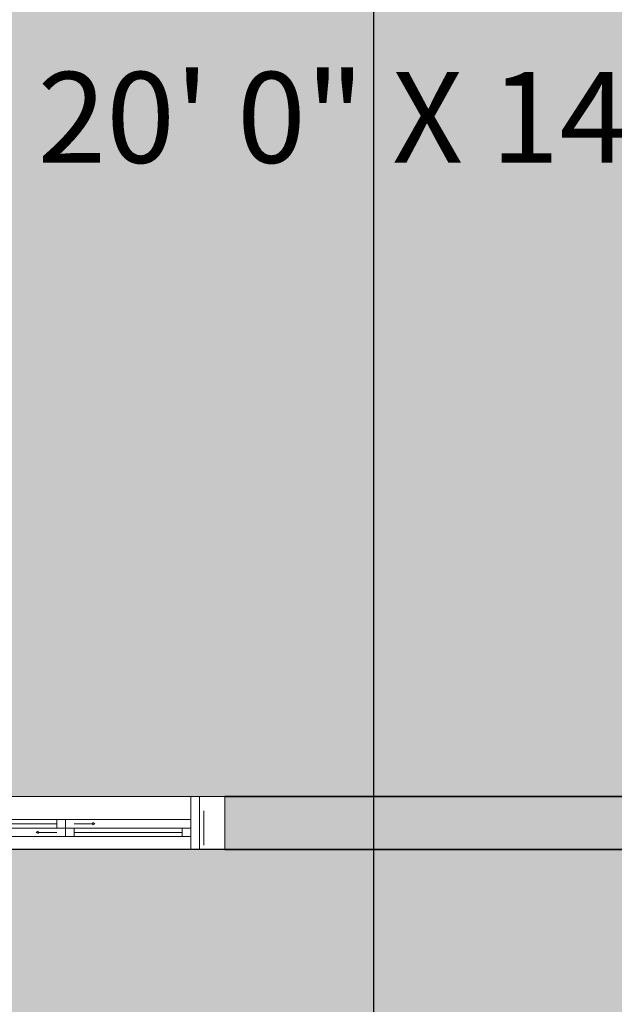
# Model space of a CAD drawing. Units: inches. Extents: x 1704 to 6393, y -157 to 1172.
# Tile 32 of 122: x 2398 to 2488, y 67 to 215. Entities that reach past the tile are written whole.
import ezdxf

# ---------------------------------------------------------------- set-up
doc = ezdxf.new("R2010")
doc.units = ezdxf.units.IN
doc.header["$MEASUREMENT"] = 0
for name, color, linetype, lineweight in [('A-ANNO-DIMS', 7, 'Continuous', 13), ('A-WALL-PATT', 7, 'Continuous', 13), ('WALLS', 7, 'Continuous', 35), ('WINDOWS', 2, 'Continuous', 18)]:
    doc.layers.add(name, color=color, linetype=linetype, lineweight=lineweight)
doc.layers.add('A-FLOR-PATT', color=7, linetype='Continuous', lineweight=13, true_color=0xf2f2f2)
doc.layers.add('L-HRDS-PATT', color=9, linetype='Continuous', lineweight=13, true_color=0xc5c1ba)
doc.styles.get("Standard").update_dxf_attribs({"font": 'arial.ttf'})
doc.dimstyles.get("Standard").update_dxf_attribs({"dimtxt": 6, "dimasz": 2, "dimexe": 0.18, "dimexo": 0.0625, "dimgap": 0.09, "dimtad": 0, "dimtih": 1, "dimtoh": 1, "dimdec": 1, "dimzin": 0, "dimdsep": 46, "dimlunit": 3, "dimtxsty": 'Standard', "dimblk": 'ARCHTICK', "dimcen": 0.09, "dimadec": 0, "dimazin": 0, "dimtfac": 1, "dimtdec": 1, "dimtofl": 0, "dimtmove": 0, "dimatfit": 3, "dimfxl": 1, "dimtolj": 1, "dimtzin": 0, "dimarcsym": 0})

# ---------------------------------------------------------------- blocks, each defined once
blk = doc.blocks.new('WIN-SLIDER-48')
for p, q in [((3.83, 8), (0, 8)), ((5.13, 8), (42.87, 8)), ((44.17, 8), (48, 8)), ((3.18, 5.86), (3.18, 0.65)), ((6.43, 4.55), (22.7, 4.55)), ((24, 4.55), (42.87, 4.55)), ((44.82, 5.86), (44.82, 0.65)), ((6.43, 3.9), (22.7, 3.9)), ((6.43, 3.25), (22.7, 3.25)), ((25.3, 3.9), (28.1, 3.9)), ((25.3, 3.25), (41.56, 3.25)), ((24, 1.95), (5.13, 1.95)), ((22.7, 2.6), (19.9, 2.6)), ((25.3, 2.6), (41.56, 2.6)), ((25.3, 1.95), (41.56, 1.95)), ((3.83, 0), (0, 0)), ((5.13, 0), (42.87, 0)), ((44.17, 0), (48, 0))]:
    blk.add_line(p, q)
for points in [[(5.13, 0), (3.83, 0), (3.83, 8), (5.13, 8)], [(42.87, 0), (44.17, 0), (44.17, 8), (42.87, 8)], [(5.13, 3.25), (6.43, 3.25), (6.43, 4.55), (5.13, 4.55)], [(22.7, 3.25), (24, 3.25), (24, 4.55), (22.7, 4.55)], [(24, 1.95), (25.3, 1.95), (25.3, 3.25), (24, 3.25)], [(28.43, 3.9), (28.1, 4.1), (28.1, 3.71)], [(41.56, 1.95), (42.87, 1.95), (42.87, 3.25), (41.56, 3.25)], [(19.57, 2.6), (19.9, 2.8), (19.9, 2.41)]]:
    blk.add_lwpolyline(points, close=True)
blk = doc.blocks.new('_ArchTick')
at = {"color": 0, "linetype": 'ByBlock', "const_width": 0.15}
blk.add_lwpolyline([(-0.5, -0.5), (0.5, 0.5)], dxfattribs=at)
blk = doc.blocks.new('*D93')
at = {"layer": 'A-ANNO-DIMS', "color": 0, "lineweight": -2, "transparency": 16777216}
for p, q in [((2605.29, 895.21), (1829.7, 895.21)), ((1829.88, 895.21), (1829.88, 495.87)), ((1829.88, 90.21), (1829.88, 489.56)), ((2605.29, 90.21), (1829.7, 90.21))]:
    blk.add_line(p, q, dxfattribs=at)
at = {"layer": 'Defpoints', "color": 0, "lineweight": -3, "transparency": 16777216}
for p in [(2605.35, 895.21), (1829.88, 90.21), (2605.35, 90.21)]:
    blk.add_point(p, dxfattribs=at)
at = {"layer": 'A-ANNO-DIMS', "color": 0, "lineweight": -2, "transparency": 16777216, "xscale": 2, "yscale": 2, "zscale": 2}
for p, rotation in [((1829.88, 895.21), 90), ((1829.88, 90.21), 270)]:
    blk.add_blockref('_ArchTick', p, dxfattribs=dict(at, rotation=rotation))
at = {"layer": 'A-ANNO-DIMS', "color": 0, "transparency": 16777216, "insert": (1829.88, 492.71), "char_height": 6, "attachment_point": 5}
blk.add_mtext('\\A1;805', dxfattribs=at)
blk = doc.blocks.new('*D105')
at = {"layer": 'A-ANNO-DIMS', "color": 0, "lineweight": -2, "transparency": 16777216}
for p, q in [((2451.74, 615.15), (2451.74, -64.97)), ((2547.35, 615.15), (2547.35, -64.97)), ((2451.74, -64.79), (2489.91, -64.79)), ((2547.35, -64.79), (2509.18, -64.79))]:
    blk.add_line(p, q, dxfattribs=at)
at = {"layer": 'Defpoints', "color": 0, "lineweight": -3, "transparency": 16777216}
for p in [(2451.74, 615.21), (2547.35, 615.21), (2547.35, -64.79)]:
    blk.add_point(p, dxfattribs=at)
at = {"layer": 'A-ANNO-DIMS', "color": 0, "lineweight": -2, "transparency": 16777216, "xscale": 2, "yscale": 2, "zscale": 2, "rotation": 180}
blk.add_blockref('_ArchTick', (2451.74, -64.79), dxfattribs=at)
at = {"layer": 'A-ANNO-DIMS', "color": 0, "lineweight": -2, "transparency": 16777216, "xscale": 2, "yscale": 2, "zscale": 2}
blk.add_blockref('_ArchTick', (2547.35, -64.79), dxfattribs=at)
at = {"layer": 'A-ANNO-DIMS', "color": 0, "transparency": 16777216, "insert": (2499.54, -64.79), "char_height": 6, "attachment_point": 5}
blk.add_mtext('\\A1;95.61', dxfattribs=at)

msp = doc.modelspace()

# ---------------------------------------------------------------- hatches: boundary and pattern name
at = {"layer": 'A-FLOR-PATT', "transparency": 33554528}
h = msp.add_hatch(color=256, dxfattribs=at)
h.dxf.hatch_style = 1
h.paths.add_polyline_path([(2325.349, 863.213), (2325.349, 887.213), (2263.349, 887.213), (2167.349, 887.213), (2081.349, 887.213), (2081.349, 719.213), (2277.349, 719.213), (2277.349, 711.213), (2277.349, 372.213), (2349.349, 372.213), (2381.349, 372.213), (2381.349, 364.213), (2353.349, 364.213), (2353.349, 270.213), (2381.349, 270.213), (2381.349, 266.213), (2357.349, 266.213), (2357.349, 98.213), (2381.349, 98.213), (2385.181, 98.213), (2386.482, 98.213), (2424.215, 98.213), (2425.516, 98.213), (2429.349, 98.213), (2597.349, 98.213), (2597.349, 146.213), (2597.349, 218.213), (2597.349, 266.213), (2423.349, 266.213), (2423.349, 270.213), (2473.349, 270.213), (2473.349, 294.213), (2477.349, 294.213), (2477.349, 270.213), (2547.349, 270.213), (2547.349, 364.213), (2477.349, 364.213), (2477.349, 318.213), (2473.349, 318.213), (2473.349, 364.213), (2423.349, 364.213), (2423.349, 372.213), (2469.349, 372.213), (2469.349, 459.213), (2469.349, 538.213), (2350.349, 538.213), (2350.349, 565.713), (2358.349, 565.713), (2358.349, 545.213), (2420.349, 545.213), (2420.349, 610.213), (2358.349, 610.213), (2358.349, 589.713), (2350.349, 589.713), (2350.349, 615.213), (2425.349, 615.213), (2425.349, 607.213), (2425.349, 546.213), (2469.349, 546.213), (2514.349, 546.213), (2514.349, 607.213), (2449.349, 607.213), (2449.349, 615.213), (2451.738, 615.213), (2451.738, 659.213), (2427.738, 659.213), (2427.738, 665.213), (2367.738, 665.213), (2367.738, 667.213), (2367.738, 711.213), (2325.349, 711.213), (2325.349, 719.213), (2325.349, 755.213), (2325.349, 763.213)])
h.paths.add_polyline_path([(2233.858, 822.533, -0.187247), (2233.858, 809.14), (2231.697, 808.804, 0.0848928), (2233.131, 814.486), (2230.424, 814.486, -0.1042581), (2228.553, 808.313), (2217.751, 807.156, -0.2222222), (2217.751, 824.517), (2228.553, 823.359, -0.1042581), (2230.424, 817.186), (2233.131, 817.186, 0.0848928), (2231.697, 822.868)], flags=16)
h.paths.add_polyline_path([(2213.621, 833.197), (2213.621, 798.475), (2156.048, 798.475), (2156.048, 833.197)], flags=16)
h.paths.add_polyline_path([(2203.932, 848.099), (2205.089, 837.296, -0.2222222), (2187.728, 837.296), (2188.885, 848.099, -0.1042581), (2195.058, 849.969), (2195.058, 852.676, 0.0848928), (2189.377, 851.242), (2189.712, 853.404, -0.187247), (2203.105, 853.404), (2203.44, 851.242, 0.0848928), (2197.759, 852.676), (2197.759, 849.969, -0.1042581)], flags=16)
h.paths.add_polyline_path([(2181.941, 837.296, -0.2222222), (2164.58, 837.296), (2165.737, 848.099, -0.1042581), (2171.91, 849.969), (2171.91, 852.676, 0.0848928), (2166.229, 851.242), (2166.564, 853.404, -0.187247), (2179.957, 853.404), (2180.292, 851.242, 0.0848928), (2174.611, 852.676), (2174.611, 849.969, -0.1042581), (2180.784, 848.099)], flags=16)
h.paths.add_polyline_path([(2205.089, 794.376), (2203.932, 783.574, -0.1042581), (2197.759, 781.703), (2197.759, 778.996, 0.0848928), (2203.44, 780.43), (2203.105, 778.269, -0.187247), (2189.712, 778.269), (2189.377, 780.43, 0.0848928), (2195.058, 778.996), (2195.058, 781.703, -0.1042581), (2188.885, 783.574), (2187.728, 794.376, -0.2222222)], flags=16)
h.paths.add_polyline_path([(2181.941, 794.376), (2180.784, 783.574, -0.1042581), (2174.611, 781.703), (2174.611, 778.996, 0.0848928), (2180.292, 780.43), (2179.957, 778.269, -0.187247), (2166.564, 778.269), (2166.229, 780.43, 0.0848928), (2171.91, 778.996), (2171.91, 781.703, -0.1042581), (2165.737, 783.574), (2164.58, 794.376, -0.2222222)], flags=16)
h.paths.add_polyline_path([(2151.918, 807.156), (2141.116, 808.313, -0.1042581), (2139.245, 814.486), (2136.539, 814.486, 0.0848928), (2137.972, 808.804), (2135.811, 809.14, -0.187247), (2135.811, 822.533), (2137.972, 822.868, 0.0848928), (2136.539, 817.186), (2139.245, 817.186, -0.1042581), (2141.116, 823.359), (2151.918, 824.517, -0.2222222)], flags=16)
h.paths.add_polyline_path([(2357.868, 363.41), (2358.814, 363.41, 0.7537605)], flags=16)
h.paths.add_polyline_path([(2372.241, 363.117), (2372.248, 363.117), (2372.248, 363.343), (2371.302, 363.343), (2371.302, 363.139, -1.3603913)], flags=16)
h.paths.add_polyline_path([(2371.309, 272.716), (2371.302, 272.716), (2371.302, 272.49), (2372.248, 272.49), (2372.248, 272.693, -1.3603913)], flags=16)
h.paths.add_polyline_path([(2357.875, 272.716), (2357.868, 272.716), (2357.868, 272.49), (2358.814, 272.49), (2358.814, 272.693, -1.3603913)], flags=16)
h.paths.add_polyline_path([(2353.769, 363.074), (2376.347, 363.074), (2376.347, 272.759), (2353.769, 272.759)], flags=16)
h.paths.add_polyline_path([(2354.772, 362.07), (2375.344, 362.07), (2375.344, 273.762), (2354.772, 273.762)], flags=0)
h.paths.add_polyline_path([(2357.868, 363.343), (2358.814, 363.343), (2358.814, 363.117), (2357.868, 363.117)], flags=16)
h.paths.add_polyline_path([(2359.288, 359.184), (2359.288, 360.063), (2370.828, 360.063), (2370.828, 359.184), (2374.332, 359.184), (2374.332, 358.464), (2372.835, 358.464), (2372.835, 357.541), (2374.332, 357.541), (2374.332, 356.82), (2372.835, 356.82), (2372.835, 355.898), (2374.332, 355.898), (2374.332, 355.177), (2372.835, 355.177), (2372.835, 354.254), (2374.332, 354.254), (2374.332, 353.534), (2372.835, 353.534), (2372.835, 352.611), (2374.332, 352.611), (2374.332, 351.89), (2372.835, 351.89), (2372.835, 350.968), (2374.332, 350.968), (2374.332, 350.247), (2372.835, 350.247), (2372.835, 349.324), (2374.332, 349.324), (2374.332, 348.604), (2372.835, 348.604), (2372.835, 347.681), (2374.332, 347.681), (2374.332, 346.96), (2372.835, 346.96), (2372.835, 346.038), (2374.332, 346.038), (2374.332, 345.317), (2372.835, 345.317), (2372.835, 344.395), (2374.332, 344.395), (2374.332, 343.674), (2372.835, 343.674), (2372.835, 342.751), (2374.332, 342.751), (2374.332, 342.03), (2372.835, 342.03), (2372.835, 341.108), (2374.332, 341.108), (2374.332, 340.387), (2372.835, 340.387), (2372.835, 339.465), (2374.332, 339.465), (2374.332, 338.744), (2372.835, 338.744), (2372.835, 337.821), (2374.332, 337.821), (2374.332, 337.1), (2372.835, 337.1), (2372.835, 336.178), (2374.332, 336.178), (2374.332, 335.457), (2372.835, 335.457), (2372.835, 334.535), (2374.332, 334.535), (2374.332, 333.814), (2372.835, 333.814), (2372.835, 332.891), (2374.332, 332.891), (2374.332, 332.171), (2372.835, 332.171), (2372.835, 331.248), (2374.332, 331.248), (2374.332, 330.527), (2372.835, 330.527), (2372.835, 329.605), (2374.332, 329.605), (2374.332, 328.884), (2372.835, 328.884), (2372.835, 327.961), (2374.332, 327.961), (2374.332, 327.241), (2372.835, 327.241), (2372.835, 326.318), (2374.332, 326.318), (2374.332, 325.597), (2372.835, 325.597), (2372.835, 324.675), (2374.332, 324.675), (2374.332, 323.954), (2372.835, 323.954), (2372.835, 323.031), (2374.332, 323.031), (2374.332, 322.311), (2372.835, 322.311), (2372.835, 321.388), (2374.332, 321.388), (2374.332, 320.667), (2372.835, 320.667), (2372.835, 319.745), (2374.332, 319.745), (2374.332, 319.024), (2372.835, 319.024), (2372.835, 318.102), (2374.332, 318.102), (2374.332, 317.381), (2372.835, 317.381), (2372.835, 316.458), (2374.332, 316.458), (2374.332, 315.737), (2372.835, 315.737), (2372.835, 314.815), (2374.332, 314.815), (2374.332, 314.094), (2372.835, 314.094), (2372.835, 313.172), (2374.332, 313.172), (2374.332, 312.451), (2372.835, 312.451), (2372.835, 311.528), (2374.332, 311.528), (2374.332, 310.807), (2372.835, 310.807), (2372.835, 309.885), (2374.332, 309.885), (2374.332, 309.164), (2372.835, 309.164), (2372.835, 308.242), (2374.332, 308.242), (2374.332, 307.521), (2372.835, 307.521), (2372.835, 306.598), (2374.332, 306.598), (2374.332, 305.878), (2372.835, 305.878), (2372.835, 304.955), (2374.332, 304.955), (2374.332, 304.234), (2372.835, 304.234), (2372.835, 303.312), (2374.332, 303.312), (2374.332, 302.591), (2372.835, 302.591), (2372.835, 301.668), (2374.332, 301.668), (2374.332, 300.948), (2372.835, 300.948), (2372.835, 300.025), (2374.332, 300.025), (2374.332, 299.304), (2372.835, 299.304), (2372.835, 298.382), (2374.332, 298.382), (2374.332, 297.661), (2372.835, 297.661), (2372.835, 296.738), (2374.332, 296.738), (2374.332, 296.018), (2372.835, 296.018), (2372.835, 295.095), (2374.332, 295.095), (2374.332, 294.374), (2372.835, 294.374), (2372.835, 293.452), (2374.332, 293.452), (2374.332, 292.731), (2372.835, 292.731), (2372.835, 291.809), (2374.332, 291.809), (2374.332, 291.088), (2372.835, 291.088), (2372.835, 290.165), (2374.332, 290.165), (2374.332, 289.444), (2372.835, 289.444), (2372.835, 288.522), (2374.332, 288.522), (2374.332, 287.801), (2372.835, 287.801), (2372.835, 286.879), (2374.332, 286.879), (2374.332, 286.158), (2372.835, 286.158), (2372.835, 285.235), (2374.332, 285.235), (2374.332, 284.514), (2372.835, 284.514), (2372.835, 283.592), (2374.332, 283.592), (2374.332, 282.871), (2372.835, 282.871), (2372.835, 281.949), (2374.332, 281.949), (2374.332, 281.228), (2372.835, 281.228), (2372.835, 280.305), (2374.332, 280.305), (2374.332, 279.585), (2372.835, 279.585), (2372.835, 278.662), (2374.332, 278.662), (2374.332, 277.941), (2372.835, 277.941), (2372.835, 277.019), (2374.332, 277.019), (2374.332, 276.298), (2370.828, 276.298), (2370.828, 275.769), (2359.288, 275.769), (2359.288, 276.298), (2355.784, 276.298), (2355.784, 277.019), (2357.281, 277.019), (2357.281, 277.941), (2355.784, 277.941), (2355.784, 278.662), (2357.281, 278.662), (2357.281, 279.585), (2355.784, 279.585), (2355.784, 280.305), (2357.281, 280.305), (2357.281, 281.228), (2355.784, 281.228), (2355.784, 281.949), (2357.281, 281.949), (2357.281, 282.871), (2355.784, 282.871), (2355.784, 283.592), (2357.281, 283.592), (2357.281, 284.514), (2355.784, 284.514), (2355.784, 285.235), (2357.281, 285.235), (2357.281, 286.158), (2355.784, 286.158), (2355.784, 286.879), (2357.281, 286.879), (2357.281, 287.801), (2355.784, 287.801), (2355.784, 288.522), (2357.281, 288.522), (2357.281, 289.444), (2355.784, 289.444), (2355.784, 290.165), (2357.281, 290.165), (2357.281, 291.088), (2355.784, 291.088), (2355.784, 291.809), (2357.281, 291.809), (2357.281, 292.731), (2355.784, 292.731), (2355.784, 293.452), (2357.281, 293.452), (2357.281, 294.374), (2355.784, 294.374), (2355.784, 295.095), (2357.281, 295.095), (2357.281, 296.018), (2355.784, 296.018), (2355.784, 296.738), (2357.281, 296.738), (2357.281, 297.661), (2355.784, 297.661), (2355.784, 298.382), (2357.281, 298.382), (2357.281, 299.304), (2355.784, 299.304), (2355.784, 300.025), (2357.281, 300.025), (2357.281, 300.948), (2355.784, 300.948), (2355.784, 301.668), (2357.281, 301.668), (2357.281, 302.591), (2355.784, 302.591), (2355.784, 303.312), (2357.281, 303.312), (2357.281, 304.234), (2355.784, 304.234), (2355.784, 304.955), (2357.281, 304.955), (2357.281, 305.878), (2355.784, 305.878), (2355.784, 306.598), (2357.281, 306.598), (2357.281, 307.521), (2355.784, 307.521), (2355.784, 308.242), (2357.281, 308.242), (2357.281, 309.164), (2355.784, 309.164), (2355.784, 309.885), (2357.281, 309.885), (2357.281, 310.807), (2355.784, 310.807), (2355.784, 311.528), (2357.281, 311.528), (2357.281, 312.451), (2355.784, 312.451), (2355.784, 313.172), (2357.281, 313.172), (2357.281, 314.094), (2355.784, 314.094), (2355.784, 314.815), (2357.281, 314.815), (2357.281, 315.737), (2355.784, 315.737), (2355.784, 316.458), (2357.281, 316.458), (2357.281, 317.381), (2355.784, 317.381), (2355.784, 318.102), (2357.281, 318.102), (2357.281, 319.024), (2355.784, 319.024), (2355.784, 319.745), (2357.281, 319.745), (2357.281, 320.667), (2355.784, 320.667), (2355.784, 321.388), (2357.281, 321.388), (2357.281, 322.311), (2355.784, 322.311), (2355.784, 323.031), (2357.281, 323.031), (2357.281, 323.954), (2355.784, 323.954), (2355.784, 324.675), (2357.281, 324.675), (2357.281, 325.597), (2355.784, 325.597), (2355.784, 326.318), (2357.281, 326.318), (2357.281, 327.241), (2355.784, 327.241), (2355.784, 327.961), (2357.281, 327.961), (2357.281, 328.884), (2355.784, 328.884), (2355.784, 329.605), (2357.281, 329.605), (2357.281, 330.527), (2355.784, 330.527), (2355.784, 331.248), (2357.281, 331.248), (2357.281, 332.171), (2355.784, 332.171), (2355.784, 332.891), (2357.281, 332.891), (2357.281, 333.814), (2355.784, 333.814), (2355.784, 334.535), (2357.281, 334.535), (2357.281, 335.457), (2355.784, 335.457), (2355.784, 336.178), (2357.281, 336.178), (2357.281, 337.1), (2355.784, 337.1), (2355.784, 337.821), (2357.281, 337.821), (2357.281, 338.744), (2355.784, 338.744), (2355.784, 339.465), (2357.281, 339.465), (2357.281, 340.387), (2355.784, 340.387), (2355.784, 341.108), (2357.281, 341.108), (2357.281, 342.03), (2355.784, 342.03), (2355.784, 342.751), (2357.281, 342.751), (2357.281, 343.674), (2355.784, 343.674), (2355.784, 344.395), (2357.281, 344.395), (2357.281, 345.317), (2355.784, 345.317), (2355.784, 346.038), (2357.281, 346.038), (2357.281, 346.96), (2355.784, 346.96), (2355.784, 347.681), (2357.281, 347.681), (2357.281, 348.604), (2355.784, 348.604), (2355.784, 349.324), (2357.281, 349.324), (2357.281, 350.247), (2355.784, 350.247), (2355.784, 350.968), (2357.281, 350.968), (2357.281, 351.89), (2355.784, 351.89), (2355.784, 352.611), (2357.281, 352.611), (2357.281, 353.534), (2355.784, 353.534), (2355.784, 354.254), (2357.281, 354.254), (2357.281, 355.177), (2355.784, 355.177), (2355.784, 355.898), (2357.281, 355.898), (2357.281, 356.82), (2355.784, 356.82), (2355.784, 357.541), (2357.281, 357.541), (2357.281, 358.464), (2355.784, 358.464), (2355.784, 359.184)], flags=0)
at = {"layer": 'A-WALL-PATT', "transparency": 33554643}
h = msp.add_hatch(color=256, dxfattribs=at)
h.dxf.hatch_style = 1
h.paths.add_polyline_path([(2167.349, 895.213), (2073.349, 895.213), (2073.349, 887.213), (2081.349, 887.213), (2167.349, 887.213)])
h.paths.add_polyline_path([(2465.349, 895.213), (2273.349, 895.213), (2273.349, 903.213), (2263.349, 903.213), (2263.349, 895.213), (2263.349, 887.213), (2325.349, 887.213), (2325.349, 863.213), (2333.349, 863.213), (2333.349, 887.213), (2465.349, 887.213)])
h.paths.add_polyline_path([(2533.349, 895.213), (2513.349, 895.213), (2513.349, 887.213), (2513.349, 861.213), (2517.349, 861.213), (2517.349, 887.213), (2533.349, 887.213)])
h.paths.add_polyline_path([(2605.349, 895.213), (2581.349, 895.213), (2581.349, 887.213), (2597.349, 887.213), (2597.349, 854.213), (2605.349, 854.213)])
h.paths.add_polyline_path([(2605.349, 752.213), (2629.349, 752.213), (2629.349, 716.213), (2605.349, 716.213), (2605.349, 712.213), (2719.349, 712.213), (2719.349, 716.213), (2631.349, 716.213), (2631.349, 754.213), (2605.349, 754.213), (2605.349, 794.213), (2597.349, 794.213), (2597.349, 787.213), (2517.349, 787.213), (2517.349, 813.213), (2513.349, 813.213), (2513.349, 783.213), (2517.349, 783.213), (2597.349, 783.213), (2597.349, 719.213), (2517.349, 719.213), (2517.349, 753.213), (2513.349, 753.213), (2513.349, 719.213), (2365.349, 719.213), (2365.349, 763.213), (2325.349, 763.213), (2325.349, 755.213), (2357.349, 755.213), (2357.349, 719.213), (2325.349, 719.213), (2325.349, 711.213), (2547.349, 711.213), (2547.349, 615.213), (2449.349, 615.213), (2449.349, 607.213), (2514.349, 607.213), (2514.349, 546.213), (2439.349, 546.213), (2425.349, 546.213), (2425.349, 607.213), (2425.349, 615.213), (2350.349, 615.213), (2350.349, 589.713), (2358.349, 589.713), (2358.349, 610.213), (2420.349, 610.213), (2420.349, 545.213), (2358.349, 545.213), (2358.349, 565.713), (2350.349, 565.713), (2350.349, 538.213), (2469.349, 538.213), (2469.349, 459.213), (2469.349, 372.213), (2423.349, 372.213), (2423.349, 364.213), (2473.349, 364.213), (2473.349, 318.213), (2477.349, 318.213), (2477.349, 364.213), (2547.349, 364.213), (2547.349, 352.213), (2549.349, 352.213), (2549.349, 364.213), (2597.349, 364.213), (2597.349, 328.213), (2549.349, 328.213), (2547.349, 328.213), (2547.349, 326.213), (2549.349, 326.213), (2597.349, 326.213), (2605.349, 326.213), (2605.349, 377.057), (2597.349, 377.057), (2597.349, 372.213), (2477.349, 372.213), (2477.349, 451.213), (2597.349, 451.213), (2605.349, 451.213), (2605.349, 459.213), (2597.349, 459.213), (2477.349, 459.213), (2477.349, 538.213), (2597.349, 538.213), (2597.349, 495.213), (2605.349, 495.213), (2605.349, 512.213), (2631.349, 512.213), (2631.349, 568.213), (2605.349, 568.213), (2605.349, 577.213), (2597.349, 577.213), (2597.349, 542.213), (2518.349, 542.213), (2518.349, 607.213), (2532.349, 607.213), (2605.349, 607.213), (2605.349, 615.213), (2597.349, 615.213), (2551.349, 615.213), (2551.349, 711.213), (2597.349, 711.213), (2597.349, 645.213), (2605.349, 645.213), (2605.349, 712.213), (2605.349, 716.213)])
h.paths.add_polyline_path([(2605.349, 566.213), (2629.349, 566.213), (2629.349, 514.213), (2605.349, 514.213)], flags=16)
h.paths.add_polyline_path([(2381.349, 372.213), (2349.349, 372.213), (2349.349, 202.213), (2337.349, 202.213), (2337.349, 194.213), (2349.349, 194.213), (2349.349, 90.213), (2349.349, 72.213), (2357.349, 72.213), (2357.349, 90.213), (2381.349, 90.213), (2381.349, 98.213), (2357.349, 98.213), (2357.349, 266.213), (2381.349, 266.213), (2381.349, 270.213), (2353.349, 270.213), (2353.349, 364.213), (2381.349, 364.213)])
h.paths.add_polyline_path([(2605.349, 302.213), (2597.349, 302.213), (2597.349, 270.213), (2477.349, 270.213), (2477.349, 294.213), (2473.349, 294.213), (2473.349, 270.213), (2423.349, 270.213), (2423.349, 266.213), (2597.349, 266.213), (2597.349, 218.213), (2605.349, 218.213)])
h.paths.add_polyline_path([(2605.349, 146.213), (2597.349, 146.213), (2597.349, 98.213), (2429.349, 98.213), (2429.349, 90.213), (2597.349, 90.213), (2597.349, 72.213), (2605.349, 72.213), (2605.349, 90.213)])
h.paths.add_polyline_path([(2225.349, 202.213), (2049.349, 202.213), (2049.349, 194.213), (2225.349, 194.213)])
h.paths.add_polyline_path([(2289.349, 202.213), (2277.349, 202.213), (2273.349, 202.213), (2269.516, 202.213), (2269.516, 194.213), (2273.349, 194.213), (2277.349, 194.213), (2289.349, 194.213)])
h.paths.add_polyline_path([(2273.349, 372.213), (2029.19, 372.213), (2029.19, 364.213), (2273.349, 364.213)])
h.paths.add_polyline_path([(2277.349, 545.213), (2213.349, 545.213), (2213.349, 573.213), (2205.349, 573.213), (2177.349, 573.213), (2177.349, 545.213), (2073.349, 545.213), (2073.349, 538.213), (2081.349, 538.213), (2277.349, 538.213)])
h.paths.add_polyline_path([(2181.349, 545.213), (2181.349, 569.213), (2205.349, 569.213), (2205.349, 545.213)], flags=16)
h.paths.add_polyline_path([(2277.349, 719.213), (2081.349, 719.213), (2073.349, 719.213), (2073.349, 711.213), (2154.575, 711.213), (2205.349, 711.213), (2205.349, 687.213), (2205.349, 629.213), (2213.349, 629.213), (2273.349, 629.213), (2273.349, 631.213), (2207.349, 631.213), (2207.349, 707.213), (2231.349, 707.213), (2231.349, 709.213), (2207.349, 709.213), (2207.349, 711.213), (2277.349, 711.213)])
at = {"layer": 'L-HRDS-PATT', "transparency": 33554539}
h = msp.add_hatch(color=256, dxfattribs=at)
h.dxf.hatch_style = 1
h.paths.add_polyline_path([(2651.217, 368.213), (2605.349, 368.213), (2605.349, 218.213), (2605.349, 212.464), (2605.349, 210.513), (2605.349, 153.913), (2605.349, 151.962), (2605.349, 146.213), (2605.349, 90.213), (2605.349, 72.213), (2601.349, 72.213), (2600.88, 50.634), (2719.349, 50.634), (2719.349, 72.213), (2711.349, 72.213), (2663.217, 72.213), (2651.217, 72.213)])
h.paths.add_polyline_path([(2711.349, 48.634), (2600.88, 48.634), (2576.88, 48.634), (2576.88, 17.658), (2711.349, 17.658)])
h.paths.add_polyline_path([(2601.349, 72.213), (2597.349, 72.213), (2597.349, 90.213), (2429.349, 90.213), (2425.516, 90.213), (2424.215, 90.213), (2386.482, 90.213), (2385.181, 90.213), (2381.349, 90.213), (2357.349, 90.213), (2357.349, 72.213), (2349.349, 72.213), (2349.349, 90.213), (2349.349, 134.213), (2277.349, 134.213), (2277.349, 50.634), (2566.88, 50.634), (2600.88, 50.634)])
h.paths.add_polyline_path([(2349.349, 146.213), (2277.349, 146.213), (2277.349, 134.213), (2349.349, 134.213)])
h.paths.add_polyline_path([(2349.349, 158.213), (2277.349, 158.213), (2277.349, 146.213), (2349.349, 146.213)])
h.paths.add_polyline_path([(2349.349, 170.213), (2277.349, 170.213), (2277.349, 158.213), (2349.349, 158.213)])
h.paths.add_polyline_path([(2349.349, 194.213), (2337.349, 194.213), (2337.349, 202.213), (2349.349, 202.213), (2349.349, 364.213), (2277.349, 364.213), (2277.349, 202.213), (2289.349, 202.213), (2289.349, 194.213), (2277.349, 194.213), (2277.349, 170.213), (2349.349, 170.213)])

# ---------------------------------------------------------------- linework, layer by layer
at = {"layer": 'WALLS'}
for p, q in [((2597.349, 98.213), (2429.349, 98.213)), ((2597.349, 90.213), (2429.349, 90.213))]:
    msp.add_line(p, q, dxfattribs=at)
at = {"layer": 'WINDOWS'}
msp.add_line((2429.349, 98.213), (2429.349, 90.213), dxfattribs=at)

# ---------------------------------------------------------------- block references
msp.add_blockref('WIN-SLIDER-48', (2381.349, 90.213), dxfattribs=at)

# ---------------------------------------------------------------- texts
at = {"layer": 'A-ANNO-DIMS'}
msp.add_text('20\' 0" X 14\' 0"', height=13.6672, dxfattribs=at).set_placement((2401.141, 193.619))

# ---------------------------------------------------------------- dimensions: what is measured, and where the dimension line sits
dim = msp.add_linear_dim(base=(1829.878, 90.213), p1=(2605.349, 895.213), p2=(2605.349, 90.213), angle=90, dimstyle='Standard', override={"dimdec": 0, "dimlfac": 1, "dimrnd": 0, "dimzin": 0, "dimdsep": 46, "dimlunit": 2}, dxfattribs=at)
dim.commit()
dim.dimension.update_dxf_attribs({"geometry": '*D93', "text_midpoint": (1829.878, 492.713)})
dim = msp.add_linear_dim(base=(2547.349, -64.787), p1=(2451.738, 615.213), p2=(2547.349, 615.213), dimstyle='Standard', override={"dimdec": 2, "dimlfac": 1, "dimrnd": 0, "dimzin": 0, "dimdsep": 46, "dimlunit": 2}, dxfattribs=at)
dim.commit()
dim.dimension.update_dxf_attribs({"geometry": '*D105', "text_midpoint": (2499.543, -64.787)})

doc.saveas('drawing.dxf')
